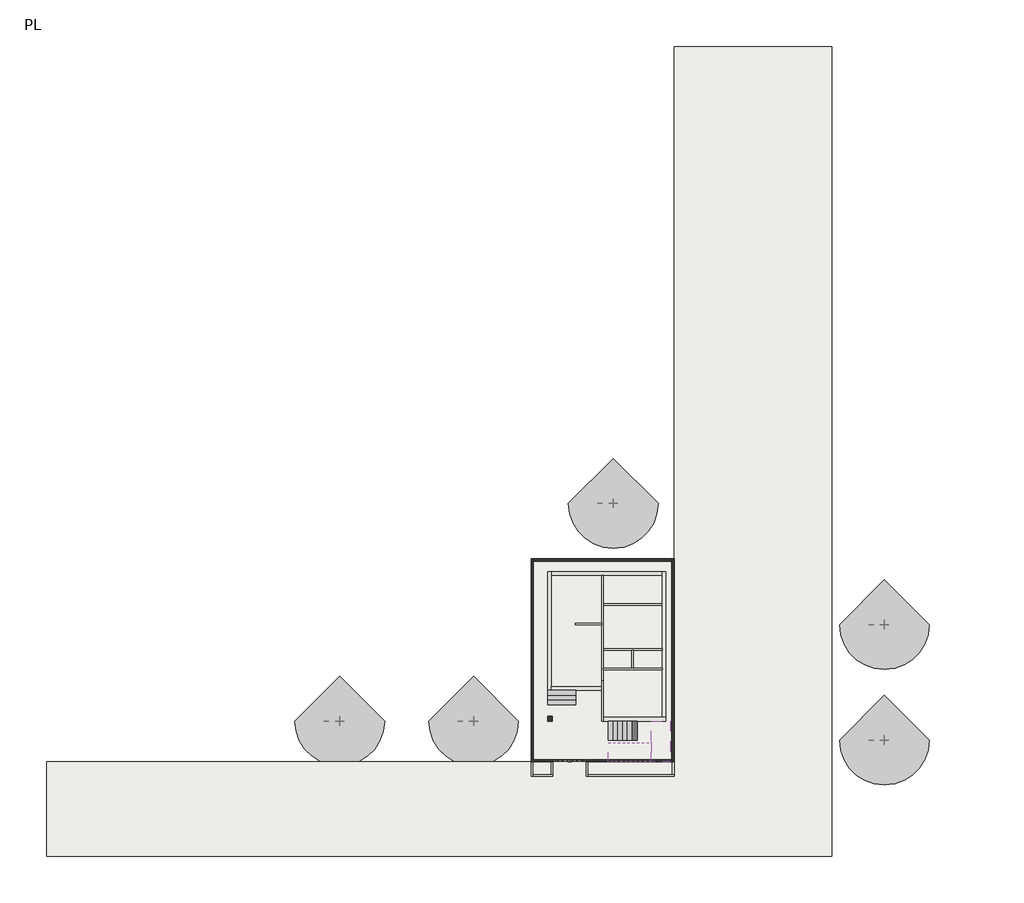
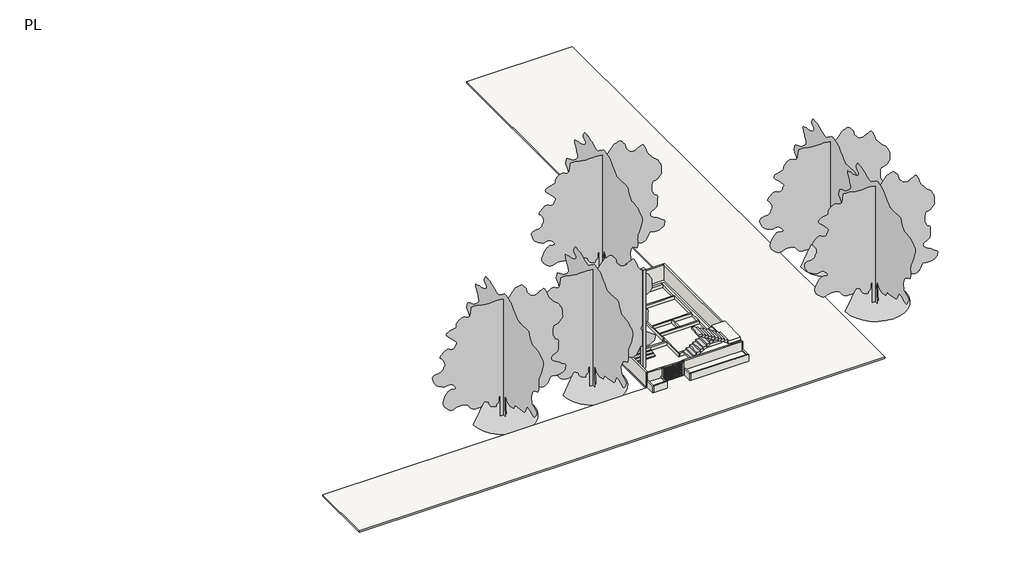
# One storey, incomplete: 23 walls, 5 geographic elements, 5 proxies, 4 slabs, 3 stair flights, 1 column.
"""IFC4 building model written with IfcOpenShell, lengths in millimetres."""

from ifc_helpers import new_model, si_unit, frame, origin, origin_with_axes, place, context, project, spatial, polyline, outline, extrude, faceted_brep, transform, mapped, element, save
from components import generic_models_1_generic_models_1_5ca79dfd, generic_models_2_generic_models_2_e4755291, generic_models_3_generic_models_1_2aceec8a, generic_models_4_generic_models_2_2859856a, generic_models_5_generic_models_5_3b624c68, m_concrete_square_column_300_x_300mm_500808f7, m_rpc_tree_fall_scarlet_oak_12_5_meters_78a4568a

model = new_model("IFC4")

# Units and contexts
model_context = context("Model", 3, world=origin())
ifc_project = project(units=[si_unit("LENGTHUNIT", "METRE", prefix="MILLI")], contexts=[model_context])

# Site, building, storey
site = spatial("IfcSite", under=ifc_project)
building = spatial("IfcBuilding", under=site)
storey = spatial("IfcBuildingStorey", under=building, Name="PL", Elevation=-457.2)

# Proxies
placement = place(None, origin())
generic_models_1_generic_models_1_shape = generic_models_1_generic_models_1_5ca79dfd(model_context)
element("IfcBuildingElementProxy", 1, Name="Generic Models 1 : Generic Models 1", ObjectType="Generic Models 1 : Generic Models 1", at=placement, inside=storey, context=model_context, shape_type="MappedRepresentation", body=[
    mapped(generic_models_1_generic_models_1_shape, transform((160.0, -777.2092348, 0.0), x_axis=(1.0, 0.0, 0.0), y_axis=(0.0, 1.0, 0.0), z_axis=(0.0, 0.0, 1.0))),
])
generic_models_2_generic_models_2_shape = generic_models_2_generic_models_2_e4755291(model_context)
element("IfcBuildingElementProxy", 2, Name="Generic Models 2 : Generic Models 2", ObjectType="Generic Models 2 : Generic Models 2", at=placement, inside=storey, context=model_context, shape_type="MappedRepresentation", body=[
    mapped(generic_models_2_generic_models_2_shape, transform((0.0, -777.2092348, 0.0), x_axis=(1.0, 0.0, 0.0), y_axis=(0.0, 1.0, 0.0), z_axis=(0.0, 0.0, 1.0))),
])
generic_models_3_generic_models_1_shape = generic_models_3_generic_models_1_2aceec8a(model_context)
element("IfcBuildingElementProxy", 3, Name="Generic Models 3 : Generic Models 1", ObjectType="Generic Models 3 : Generic Models 1", at=placement, inside=storey, context=model_context, shape_type="MappedRepresentation", body=[
    mapped(generic_models_3_generic_models_1_shape, transform((152.4, -777.2092348, 0.0), x_axis=(1.0, 0.0, 0.0), y_axis=(0.0, 1.0, 0.0), z_axis=(0.0, 0.0, 1.0))),
])
generic_models_4_generic_models_2_shape = generic_models_4_generic_models_2_2859856a(model_context)
element("IfcBuildingElementProxy", 4, Name="Generic Models 4 : Generic Models 2", ObjectType="Generic Models 4 : Generic Models 2", at=placement, inside=storey, context=model_context, shape_type="MappedRepresentation", body=[
    mapped(generic_models_4_generic_models_2_shape, transform((140.0, -777.2092348, 0.0), x_axis=(1.0, 0.0, 0.0), y_axis=(0.0, 1.0, 0.0), z_axis=(0.0, 0.0, 1.0))),
])
generic_models_5_generic_models_5_shape = generic_models_5_generic_models_5_3b624c68(model_context)
element("IfcBuildingElementProxy", 5, Name="Generic Models 5 : Generic Models 5", ObjectType="Generic Models 5 : Generic Models 5", at=placement, inside=storey, context=model_context, shape_type="MappedRepresentation", body=[
    mapped(generic_models_5_generic_models_5_shape, transform((0.0, 0.0, 0.0), x_axis=(1.0, 0.0, 0.0), y_axis=(0.0, 1.0, 0.0), z_axis=(0.0, 0.0, 1.0))),
])

# Column
m_concrete_square_column_300_x_300mm_shape = m_concrete_square_column_300_x_300mm_500808f7(model_context)
element("IfcColumn", 6, ObjectType="M_Concrete-Square-Column : 300 x 300mm", at=placement, inside=storey, context=model_context, shape_type="MappedRepresentation", body=[
    mapped(m_concrete_square_column_300_x_300mm_shape, transform((-3494.8544048, -4265.8648653, 0.0), x_axis=(1.0, 0.0, 0.0), y_axis=(0.0, 1.0, 0.0), z_axis=(0.0, 0.0, 1.0))),
])

# Geographic elements
m_rpc_tree_fall_scarlet_oak_12_5_meters_shape = m_rpc_tree_fall_scarlet_oak_12_5_meters_78a4568a(model_context)
element("IfcGeographicElement", 7, ObjectType="M_RPC Tree - Fall : Scarlet Oak - 12.5 Meters", at=placement, inside=storey, context=model_context, shape_type="MappedRepresentation", body=[
    mapped(m_rpc_tree_fall_scarlet_oak_12_5_meters_shape, transform((-8369.2544048, -4415.8648653, -457.2), x_axis=(1.0, 0.0, 0.0), y_axis=(0.0, 1.0, 0.0), z_axis=(0.0, 0.0, 1.0))),
])
element("IfcGeographicElement", 8, ObjectType="M_RPC Tree - Fall : Scarlet Oak - 12.5 Meters", at=placement, inside=storey, context=model_context, shape_type="MappedRepresentation", body=[
    mapped(m_rpc_tree_fall_scarlet_oak_12_5_meters_shape, transform((-16903.6544048, -4415.8648653, -457.2), x_axis=(1.0, 0.0, 0.0), y_axis=(0.0, 1.0, 0.0), z_axis=(0.0, 0.0, 1.0))),
])
element("IfcGeographicElement", 9, ObjectType="M_RPC Tree - Fall : Scarlet Oak - 12.5 Meters", at=placement, inside=storey, context=model_context, shape_type="MappedRepresentation", body=[
    mapped(m_rpc_tree_fall_scarlet_oak_12_5_meters_shape, transform((17818.1455952, -5635.0648653, -457.2), x_axis=(1.0, 0.0, 0.0), y_axis=(0.0, 1.0, 0.0), z_axis=(0.0, 0.0, 1.0))),
])
element("IfcGeographicElement", 10, ObjectType="M_RPC Tree - Fall : Scarlet Oak - 12.5 Meters", at=placement, inside=storey, context=model_context, shape_type="MappedRepresentation", body=[
    mapped(m_rpc_tree_fall_scarlet_oak_12_5_meters_shape, transform((17818.1455952, 1730.9351347, -457.2), x_axis=(1.0, 0.0, 0.0), y_axis=(0.0, 1.0, 0.0), z_axis=(0.0, 0.0, 1.0))),
])
element("IfcGeographicElement", 11, ObjectType="M_RPC Tree - Fall : Scarlet Oak - 12.5 Meters", at=placement, inside=storey, context=model_context, shape_type="MappedRepresentation", body=[
    mapped(m_rpc_tree_fall_scarlet_oak_12_5_meters_shape, transform((532.9027938, 9457.3072301, -457.2), x_axis=(1.0, 0.0, 0.0), y_axis=(0.0, 1.0, 0.0), z_axis=(0.0, 0.0, 1.0))),
])

# Slabs
element("IfcSlab", 12, ObjectType="300mm Thickness", at=placement, inside=storey, context=model_context, shape_type="Brep", body=[
    faceted_brep([(2959.1455952, -4415.8648653, 1612.2315789), (2959.1455952, -5635.0648653, 1612.2315789), (2959.1455952, -5787.4648653, 1612.2315789), (2959.1455952, -7006.6648653, 1612.2315789), (3177.9478897, -7006.6648653, 1612.2315789), (4178.3455952, -7006.6648653, 1612.2315789), (4178.3455952, -4415.8648653, 1612.2315789), (3045.1433006, -4415.8648653, 1612.2315789), (2959.1455952, -4415.8648653, 1435.7684211), (2959.1455952, -4415.8648653, 1262.4434337), (2959.1455952, -5635.0648653, 1262.4434337), (2959.1455952, -5635.0648653, 1312.2315789), (2959.1455952, -5787.4648653, 1312.2315789), (2959.1455952, -5787.4648653, 1438.9065916), (2959.1455952, -7006.6648653, 1438.9065916), (3177.9478897, -7006.6648653, 1312.2315789), (4178.3455952, -7006.6648653, 1312.2315789), (4178.3455952, -4415.8648653, 1312.2315789), (3045.1433006, -4415.8648653, 1312.2315789), (3177.9478897, -5787.4648653, 1312.2315789), (3045.1433006, -5635.0648653, 1312.2315789)], [[[0, 1, 2, 3, 4, 5, 6, 7]], [[1, 0, 8, 9, 10, 11]], [[2, 1, 11, 12, 13]], [[3, 2, 13, 14]], [[3, 14, 15, 16, 5, 4]], [[6, 5, 16, 17]], [[9, 8, 0, 7, 6, 17, 18]], [[19, 12, 11, 20, 18, 17, 16, 15]], [[12, 19, 13]], [[18, 20, 10, 9]], [[20, 11, 10]], [[19, 15, 14, 13]]]),
])
element("IfcSlab", 13, ObjectType="6\" floor", at=placement, inside=storey, context=model_context, shape_type="SweptSolid", body=[
    extrude(outline(polyline([(4406.9455952, 5921.9351347), (4406.9455952, -7021.8741001), (-4711.6544048, -7021.8741001), (-4711.6544048, 5921.9351347), (4406.9455952, 5921.9351347)])), frame((0.0, 0.0, -609.6), z_axis=(0.0, 0.0, 1.0), x_axis=(1.0, 0.0, 0.0)), (0.0, 0.0, 1.0), 152.4),
])
element("IfcSlab", 14, ObjectType="6\" floor", at=placement, inside=storey, context=model_context, shape_type="SweptSolid", body=[
    extrude(outline(polyline([(4406.9455952, -7021.8741001), (4406.9455952, 38578.1258999), (14465.3455952, 38578.1258999), (14465.3455952, -5401.8741001), (14465.3455952, -13021.8741001), (-35593.0544048, -13021.8741001), (-35593.0544048, -7021.8741001), (4406.9455952, -7021.8741001)])), frame((0.0, 0.0, -533.4), z_axis=(0.0, 0.0, 1.0), x_axis=(1.0, 0.0, 0.0)), (0.0, 0.0, 1.0), 152.4),
])
element("IfcSlab", 15, ObjectType="6\" floor 2", at=placement, inside=storey, context=model_context, shape_type="SweptSolid", body=[
    extrude(outline(polyline([(-3416.2544048, -7021.8741001), (-3416.2544048, -7834.6741001), (-4610.0544048, -7834.6741001), (-4610.0544048, -7021.8741001), (-3416.2544048, -7021.8741001)])), origin_with_axes(), (0.0, 0.0, 1.0), 152.4),
    extrude(outline(polyline([(4305.3455952, -7021.8741001), (4305.3455952, -7834.6741001), (-1079.4544048, -7834.6741001), (-1079.4544048, -7021.8741001), (4305.3455952, -7021.8741001)])), origin_with_axes(), (0.0, 0.0, 1.0), 152.4),
])

# Stair flights
element("IfcStairFlight", 16, ObjectType="150mm Depth", at=placement, inside=storey, context=model_context, shape_type="Brep", body=[
    faceted_brep([(-3644.8544048, -3069.6648653, -342.9), (-3644.8544048, -3374.4648653, -342.9), (-1854.2524777, -3374.4648653, -342.9), (-1854.2524777, -3069.6648653, -342.9), (-3644.8544048, -3069.6648653, -457.2), (-3644.8544048, -3374.4648653, -457.2), (-1854.2524777, -3374.4648653, -457.2), (-1854.2524777, -3069.6648653, -457.2), (-3644.8544048, -2764.8648653, -228.6), (-3644.8544048, -3069.6648653, -228.6), (-1854.2524777, -3069.6648653, -228.6), (-1854.2524777, -2764.8648653, -228.6), (-3644.8544048, -2764.8648653, -388.8000702), (-3644.8544048, -2947.264678, -457.2), (-1854.2524777, -2947.264678, -457.2), (-1854.2524777, -2764.8648653, -388.8000702), (-3644.8544048, -2460.0648653, -114.3), (-3644.8544048, -2764.8648653, -114.3), (-1854.2524777, -2764.8648653, -114.3), (-1854.2524777, -2460.0648653, -114.3), (-3644.8544048, -2460.0648653, -274.5000702), (-1854.2524777, -2460.0648653, -274.5000702)], [[[0, 1, 2, 3]], [[1, 0, 4, 5]], [[2, 1, 5, 6]], [[3, 2, 6, 7]], [[8, 9, 10, 11]], [[4, 0, 9, 8, 12, 13]], [[0, 3, 10, 9]], [[3, 7, 14, 15, 11, 10]], [[16, 17, 18, 19]], [[17, 16, 20, 12, 8]], [[8, 11, 18, 17]], [[19, 18, 11, 15, 21]], [[16, 19, 21, 20]], [[5, 4, 13, 14, 7, 6]], [[14, 13, 12, 20, 21, 15]]]),
])
element("IfcStairFlight", 17, ObjectType="150mm Depth", at=placement, inside=storey, context=model_context, shape_type="Brep", body=[
    faceted_brep([(520.7455952, -4415.8648653, 24.0631579), (215.9455952, -4415.8648653, 24.0631579), (215.9455952, -5635.0648653, 24.0631579), (520.7455952, -5635.0648653, 24.0631579), (520.7455952, -4415.8648653, -149.2618295), (515.3251188, -4415.8648653, -152.4), (215.9455952, -4415.8648653, -152.4), (215.9455952, -5635.0648653, -152.4), (515.3251188, -5635.0648653, -152.4), (520.7455952, -5635.0648653, -149.2618295), (825.5455952, -4415.8648653, 200.5263158), (520.7455952, -4415.8648653, 200.5263158), (520.7455952, -5635.0648653, 200.5263158), (825.5455952, -5635.0648653, 200.5263158), (825.5455952, -4415.8648653, 27.2013284), (825.5455952, -5635.0648653, 27.2013284), (1130.3455952, -4415.8648653, 376.9894737), (825.5455952, -4415.8648653, 376.9894737), (825.5455952, -5635.0648653, 376.9894737), (1130.3455952, -5635.0648653, 376.9894737), (1130.3455952, -4415.8648653, 203.6644863), (1130.3455952, -5635.0648653, 203.6644863), (1435.1455952, -4415.8648653, 553.4526316), (1130.3455952, -4415.8648653, 553.4526316), (1130.3455952, -5635.0648653, 553.4526316), (1435.1455952, -5635.0648653, 553.4526316), (1435.1455952, -4415.8648653, 380.1276442), (1435.1455952, -5635.0648653, 380.1276442), (1739.9455952, -4415.8648653, 729.9157895), (1435.1455952, -4415.8648653, 729.9157895), (1435.1455952, -5635.0648653, 729.9157895), (1739.9455952, -5635.0648653, 729.9157895), (1739.9455952, -4415.8648653, 556.5908021), (1739.9455952, -5635.0648653, 556.5908021), (2044.7455952, -4415.8648653, 906.3789474), (1739.9455952, -4415.8648653, 906.3789474), (1739.9455952, -5635.0648653, 906.3789474), (2044.7455952, -5635.0648653, 906.3789474), (2044.7455952, -4415.8648653, 733.05396), (2044.7455952, -5635.0648653, 733.05396), (2349.5455952, -4415.8648653, 1082.8421053), (2044.7455952, -4415.8648653, 1082.8421053), (2044.7455952, -5635.0648653, 1082.8421053), (2349.5455952, -5635.0648653, 1082.8421053), (2349.5455952, -4415.8648653, 909.5171179), (2349.5455952, -5635.0648653, 909.5171179), (2654.3455952, -4415.8648653, 1259.3052632), (2349.5455952, -4415.8648653, 1259.3052632), (2349.5455952, -5635.0648653, 1259.3052632), (2654.3455952, -5635.0648653, 1259.3052632), (2654.3455952, -4415.8648653, 1085.9802758), (2654.3455952, -5635.0648653, 1085.9802758), (2959.1455952, -4415.8648653, 1435.7684211), (2654.3455952, -4415.8648653, 1435.7684211), (2654.3455952, -5635.0648653, 1435.7684211), (2959.1455952, -5635.0648653, 1435.7684211), (2959.1455952, -4415.8648653, 1262.4434337), (2959.1455952, -5635.0648653, 1262.4434337), (2959.1455952, -5635.0648653, 1312.2315789)], [[[0, 1, 2, 3]], [[1, 0, 4, 5, 6]], [[2, 1, 6, 7]], [[3, 2, 7, 8, 9]], [[10, 11, 12, 13]], [[11, 10, 14, 4, 0]], [[0, 3, 12, 11]], [[13, 12, 3, 9, 15]], [[16, 17, 18, 19]], [[17, 16, 20, 14, 10]], [[10, 13, 18, 17]], [[19, 18, 13, 15, 21]], [[22, 23, 24, 25]], [[23, 22, 26, 20, 16]], [[16, 19, 24, 23]], [[25, 24, 19, 21, 27]], [[28, 29, 30, 31]], [[29, 28, 32, 26, 22]], [[22, 25, 30, 29]], [[31, 30, 25, 27, 33]], [[34, 35, 36, 37]], [[35, 34, 38, 32, 28]], [[28, 31, 36, 35]], [[37, 36, 31, 33, 39]], [[40, 41, 42, 43]], [[41, 40, 44, 38, 34]], [[34, 37, 42, 41]], [[43, 42, 37, 39, 45]], [[46, 47, 48, 49]], [[47, 46, 50, 44, 40]], [[40, 43, 48, 47]], [[49, 48, 43, 45, 51]], [[52, 53, 54, 55]], [[53, 52, 56, 50, 46]], [[46, 49, 54, 53]], [[55, 54, 49, 51, 57, 58]], [[52, 55, 58, 57, 56]], [[7, 6, 5, 8]], [[8, 5, 4, 14, 20, 26, 32, 38, 44, 50, 56, 57, 51, 45, 39, 33, 27, 21, 15, 9]]]),
])
element("IfcStairFlight", 18, ObjectType="150mm Depth", at=placement, inside=storey, context=model_context, shape_type="Brep", body=[
    faceted_brep([(2654.3455952, -7006.6648653, 1788.6947368), (2959.1455952, -7006.6648653, 1788.6947368), (2959.1455952, -5787.4648653, 1788.6947368), (2654.3455952, -5787.4648653, 1788.6947368), (2654.3455952, -7006.6648653, 1615.3697495), (2959.1455952, -7006.6648653, 1438.9065916), (2959.1455952, -7006.6648653, 1612.2315789), (2959.1455952, -5787.4648653, 1438.9065916), (2654.3455952, -5787.4648653, 1615.3697495), (2349.5455952, -7006.6648653, 1965.1578947), (2654.3455952, -7006.6648653, 1965.1578947), (2654.3455952, -5787.4648653, 1965.1578947), (2349.5455952, -5787.4648653, 1965.1578947), (2349.5455952, -7006.6648653, 1791.8329074), (2349.5455952, -5787.4648653, 1791.8329074), (2044.7455952, -7006.6648653, 2141.6210526), (2349.5455952, -7006.6648653, 2141.6210526), (2349.5455952, -5787.4648653, 2141.6210526), (2044.7455952, -5787.4648653, 2141.6210526), (2044.7455952, -7006.6648653, 1968.2960653), (2044.7455952, -5787.4648653, 1968.2960653), (1739.9455952, -7006.6648653, 2318.0842105), (2044.7455952, -7006.6648653, 2318.0842105), (2044.7455952, -5787.4648653, 2318.0842105), (1739.9455952, -5787.4648653, 2318.0842105), (1739.9455952, -7006.6648653, 2144.7592232), (1739.9455952, -5787.4648653, 2144.7592232), (1435.1455952, -7006.6648653, 2494.5473684), (1739.9455952, -7006.6648653, 2494.5473684), (1739.9455952, -5787.4648653, 2494.5473684), (1435.1455952, -5787.4648653, 2494.5473684), (1435.1455952, -7006.6648653, 2321.2223811), (1435.1455952, -5787.4648653, 2321.2223811), (1130.3455952, -7006.6648653, 2671.0105263), (1435.1455952, -7006.6648653, 2671.0105263), (1435.1455952, -5787.4648653, 2671.0105263), (1130.3455952, -5787.4648653, 2671.0105263), (1130.3455952, -7006.6648653, 2497.6855389), (1130.3455952, -5787.4648653, 2497.6855389), (825.5455952, -7006.6648653, 2847.4736842), (1130.3455952, -7006.6648653, 2847.4736842), (1130.3455952, -5787.4648653, 2847.4736842), (825.5455952, -5787.4648653, 2847.4736842), (825.5455952, -7006.6648653, 2674.1486968), (825.5455952, -5787.4648653, 2674.1486968), (520.7455952, -7006.6648653, 3023.9368421), (825.5455952, -7006.6648653, 3023.9368421), (825.5455952, -5787.4648653, 3023.9368421), (520.7455952, -5787.4648653, 3023.9368421), (520.7455952, -7006.6648653, 2850.6118547), (520.7455952, -5787.4648653, 2850.6118547), (215.9455952, -7006.6648653, 3200.4), (520.7455952, -7006.6648653, 3200.4), (520.7455952, -5787.4648653, 3200.4), (215.9455952, -5787.4648653, 3200.4), (215.9455952, -7006.6648653, 3027.0750126), (215.9455952, -5787.4648653, 3027.0750126)], [[[0, 1, 2, 3]], [[1, 0, 4, 5, 6]], [[2, 1, 6, 5, 7]], [[3, 2, 7, 8]], [[9, 10, 11, 12]], [[10, 9, 13, 4, 0]], [[11, 10, 0, 3]], [[12, 11, 3, 8, 14]], [[15, 16, 17, 18]], [[16, 15, 19, 13, 9]], [[17, 16, 9, 12]], [[18, 17, 12, 14, 20]], [[21, 22, 23, 24]], [[22, 21, 25, 19, 15]], [[23, 22, 15, 18]], [[24, 23, 18, 20, 26]], [[27, 28, 29, 30]], [[28, 27, 31, 25, 21]], [[29, 28, 21, 24]], [[30, 29, 24, 26, 32]], [[33, 34, 35, 36]], [[34, 33, 37, 31, 27]], [[35, 34, 27, 30]], [[36, 35, 30, 32, 38]], [[39, 40, 41, 42]], [[40, 39, 43, 37, 33]], [[41, 40, 33, 36]], [[42, 41, 36, 38, 44]], [[45, 46, 47, 48]], [[46, 45, 49, 43, 39]], [[47, 46, 39, 42]], [[48, 47, 42, 44, 50]], [[51, 52, 53, 54]], [[52, 51, 55, 49, 45]], [[53, 52, 45, 48]], [[54, 53, 48, 50, 56]], [[51, 54, 56, 55]], [[5, 4, 13, 19, 25, 31, 37, 43, 49, 55, 56, 50, 44, 38, 32, 26, 20, 14, 8, 7]]]),
])

# Walls
element("IfcWall", 19, ObjectType="4\" wall", at=placement, inside=storey, context=model_context, shape_type="Brep", body=[
    faceted_brep([(-215.8544048, -1845.1648653, -457.2), (-215.8544048, -2231.4648653, -457.2), (-215.8544048, -2460.0648653, -457.2), (-215.8544048, -4415.8648653, -457.2), (-215.8544048, -4415.8648653, -152.4), (-215.8544048, -2460.0648653, -152.4), (-215.8544048, -2231.4648653, -152.4), (-215.8544048, -1845.1648653, -152.4), (-114.2544048, -1845.1648653, -457.2), (-114.2544048, -1845.1648653, -152.4), (-114.2544048, -4187.2648653, -152.4), (-114.2544048, -4415.8648653, -152.4), (-114.2544048, -4415.8648653, -457.2), (-114.2544048, -4187.2648653, -457.2)], [[[0, 1, 2, 3, 4, 5, 6, 7]], [[8, 9, 10, 11, 12, 13]], [[3, 2, 1, 0, 8, 13, 12]], [[7, 6, 5, 4, 11, 10, 9]], [[0, 7, 9, 8]], [[4, 3, 12, 11]]]),
])
element("IfcWall", 20, ObjectType="4\" wall", at=placement, inside=storey, context=model_context, shape_type="Brep", body=[
    faceted_brep([(-215.8544048, 4880.5351347, -457.2), (-215.8544048, 1832.5351347, -457.2), (-215.8544048, 1730.9351347, -457.2), (-215.8544048, -1845.1648653, -457.2), (-215.8544048, -1845.1648653, -152.4), (-215.8544048, 1730.9351347, -152.4), (-215.8544048, 1832.5351347, -152.4), (-215.8544048, 4880.5351347, -152.4), (-114.2544048, 4880.5351347, -457.2), (-114.2544048, 4880.5351347, -152.4), (-114.2544048, 3051.7351347, -152.4), (-114.2544048, 2950.1351347, -152.4), (-114.2544048, 206.9351347, -152.4), (-114.2544048, 105.3351347, -152.4), (-114.2544048, -1037.6648653, -152.4), (-114.2544048, -1139.2648653, -152.4), (-114.2544048, -1845.1648653, -152.4), (-114.2544048, -1845.1648653, -457.2), (-114.2544048, -1139.2648653, -457.2), (-114.2544048, -1037.6648653, -457.2), (-114.2544048, 105.3351347, -457.2), (-114.2544048, 206.9351347, -457.2), (-114.2544048, 2950.1351347, -457.2), (-114.2544048, 3051.7351347, -457.2)], [[[0, 1, 2, 3, 4, 5, 6, 7]], [[8, 9, 10, 11, 12, 13, 14, 15, 16, 17, 18, 19, 20, 21, 22, 23]], [[3, 2, 1, 0, 8, 23, 22, 21, 20, 19, 18, 17]], [[4, 3, 17, 16]], [[7, 6, 5, 4, 16, 15, 14, 13, 12, 11, 10, 9]], [[0, 7, 9, 8]]]),
])
element("IfcWall", 21, ObjectType="4\" wall", at=placement, inside=storey, context=model_context, shape_type="Brep", body=[
    faceted_brep([(-114.2544048, -1139.2648653, -457.2), (3644.9455952, -1139.2648653, -457.2), (3644.9455952, -1139.2648653, -152.4), (-114.2544048, -1139.2648653, -152.4), (-114.2544048, -1037.6648653, -457.2), (-114.2544048, -1037.6648653, -152.4), (1714.5455952, -1037.6648653, -152.4), (1816.1455952, -1037.6648653, -152.4), (3644.9455952, -1037.6648653, -152.4), (3644.9455952, -1037.6648653, -457.2), (1816.1455952, -1037.6648653, -457.2), (1714.5455952, -1037.6648653, -457.2)], [[[0, 1, 2, 3]], [[4, 5, 6, 7, 8, 9, 10, 11]], [[1, 0, 4, 11, 10, 9]], [[3, 2, 8, 7, 6, 5]], [[2, 1, 9, 8]], [[0, 3, 5, 4]]]),
])
element("IfcWall", 22, ObjectType="4\" wall", at=placement, inside=storey, context=model_context, shape_type="Brep", body=[
    faceted_brep([(3644.9455952, 206.9351347, -457.2), (-114.2544048, 206.9351347, -457.2), (-114.2544048, 206.9351347, -152.4), (3644.9455952, 206.9351347, -152.4), (3644.9455952, 105.3351347, -457.2), (3644.9455952, 105.3351347, -152.4), (1816.1455952, 105.3351347, -152.4), (1714.5455952, 105.3351347, -152.4), (-114.2544048, 105.3351347, -152.4), (-114.2544048, 105.3351347, -457.2), (1714.5455952, 105.3351347, -457.2), (1816.1455952, 105.3351347, -457.2)], [[[0, 1, 2, 3]], [[4, 5, 6, 7, 8, 9, 10, 11]], [[1, 0, 4, 11, 10, 9]], [[3, 2, 8, 7, 6, 5]], [[0, 3, 5, 4]], [[2, 1, 9, 8]]]),
])
element("IfcWall", 23, ObjectType="4\" wall", at=placement, inside=storey, context=model_context, shape_type="SweptSolid", body=[
    extrude(outline(polyline([(-215.8544048, 1730.9351347), (-1892.2544048, 1730.9351347), (-1892.2544048, 1832.5351347), (-215.8544048, 1832.5351347), (-215.8544048, 1730.9351347)])), frame((0.0, 0.0, -457.2), z_axis=(0.0, 0.0, 1.0), x_axis=(1.0, 0.0, 0.0)), (0.0, 0.0, 1.0), 304.8),
])
element("IfcWall", 24, ObjectType="4\" wall", at=placement, inside=storey, context=model_context, shape_type="SweptSolid", body=[
    extrude(outline(polyline([(-114.2544048, 3051.7351347), (3644.9455952, 3051.7351347), (3644.9455952, 2950.1351347), (-114.2544048, 2950.1351347), (-114.2544048, 3051.7351347)])), frame((0.0, 0.0, -457.2), z_axis=(0.0, 0.0, 1.0), x_axis=(1.0, 0.0, 0.0)), (0.0, 0.0, 1.0), 304.8),
])
element("IfcWall", 25, ObjectType="4\" wall", at=placement, inside=storey, context=model_context, shape_type="SweptSolid", body=[
    extrude(outline(polyline([(1714.5455952, -1037.6648653), (1714.5455952, 105.3351347), (1816.1455952, 105.3351347), (1816.1455952, -1037.6648653), (1714.5455952, -1037.6648653)])), frame((0.0, 0.0, -457.2), z_axis=(0.0, 0.0, 1.0), x_axis=(1.0, 0.0, 0.0)), (0.0, 0.0, 1.0), 304.8),
])
element("IfcWall", 26, ObjectType="4\" wall", at=placement, inside=storey, context=model_context, shape_type="Brep", body=[
    faceted_brep([(-4711.6544048, -7021.8741001, -457.2), (-4711.6544048, -7936.2741001, -457.2), (-4711.6544048, -7936.2741001, 304.8), (-4711.6544048, -7021.8741001, 304.8), (-4610.0544048, -7021.8741001, -457.2), (-4610.0544048, -7021.8741001, 304.8), (-4610.0544048, -7834.6741001, 304.8), (-4610.0544048, -7936.2741001, 304.8), (-4610.0544048, -7936.2741001, -457.2), (-4610.0544048, -7834.6741001, -457.2)], [[[0, 1, 2, 3]], [[4, 5, 6, 7, 8, 9]], [[1, 0, 4, 9, 8]], [[3, 2, 7, 6, 5]], [[0, 3, 5, 4]], [[2, 1, 8, 7]]]),
])
element("IfcWall", 27, ObjectType="4\" wall", at=placement, inside=storey, context=model_context, shape_type="Brep", body=[
    faceted_brep([(-4610.0544048, -7936.2741001, -457.2), (-3314.6544048, -7936.2741001, -457.2), (-3314.6544048, -7936.2741001, 304.8), (-4610.0544048, -7936.2741001, 304.8), (-4610.0544048, -7834.6741001, -457.2), (-4610.0544048, -7834.6741001, 304.8), (-3416.2544048, -7834.6741001, 304.8), (-3314.6544048, -7834.6741001, 304.8), (-3314.6544048, -7834.6741001, -457.2), (-3416.2544048, -7834.6741001, -457.2)], [[[0, 1, 2, 3]], [[4, 5, 6, 7, 8, 9]], [[1, 0, 4, 9, 8]], [[3, 2, 7, 6, 5]], [[0, 3, 5, 4]], [[2, 1, 8, 7]]]),
])
element("IfcWall", 28, ObjectType="4\" wall", at=placement, inside=storey, context=model_context, shape_type="SweptSolid", body=[
    extrude(outline(polyline([(-3314.6544048, -7021.8741001), (-3314.6544048, -7834.6741001), (-3416.2544048, -7834.6741001), (-3416.2544048, -7021.8741001), (-3314.6544048, -7021.8741001)])), frame((0.0, 0.0, -457.2), z_axis=(0.0, 0.0, 1.0), x_axis=(1.0, 0.0, 0.0)), (0.0, 0.0, 1.0), 762.0),
])
element("IfcWall", 29, ObjectType="4\" wall", at=placement, inside=storey, context=model_context, shape_type="Brep", body=[
    faceted_brep([(-1181.0544048, -7021.8741001, -457.2), (-1181.0544048, -7936.2741001, -457.2), (-1181.0544048, -7936.2741001, 304.8), (-1181.0544048, -7021.8741001, 304.8), (-1079.4544048, -7021.8741001, -457.2), (-1079.4544048, -7021.8741001, 304.8), (-1079.4544048, -7834.6741001, 304.8), (-1079.4544048, -7936.2741001, 304.8), (-1079.4544048, -7936.2741001, -457.2), (-1079.4544048, -7834.6741001, -457.2)], [[[0, 1, 2, 3]], [[4, 5, 6, 7, 8, 9]], [[1, 0, 4, 9, 8]], [[3, 2, 7, 6, 5]], [[0, 3, 5, 4]], [[2, 1, 8, 7]]]),
])
element("IfcWall", 30, ObjectType="4\" wall", at=placement, inside=storey, context=model_context, shape_type="Brep", body=[
    faceted_brep([(-1079.4544048, -7936.2741001, -457.2), (4406.9455952, -7936.2741001, -457.2), (4406.9455952, -7936.2741001, 304.8), (-1079.4544048, -7936.2741001, 304.8), (-1079.4544048, -7834.6741001, -457.2), (-1079.4544048, -7834.6741001, 304.8), (4305.3455952, -7834.6741001, 304.8), (4406.9455952, -7834.6741001, 304.8), (4406.9455952, -7834.6741001, -457.2), (4305.3455952, -7834.6741001, -457.2)], [[[0, 1, 2, 3]], [[4, 5, 6, 7, 8, 9]], [[1, 0, 4, 9, 8]], [[3, 2, 7, 6, 5]], [[0, 3, 5, 4]], [[2, 1, 8, 7]]]),
])
element("IfcWall", 31, ObjectType="4\" wall", at=placement, inside=storey, context=model_context, shape_type="SweptSolid", body=[
    extrude(outline(polyline([(4406.9455952, -7021.8741001), (4406.9455952, -7834.6741001), (4305.3455952, -7834.6741001), (4305.3455952, -7021.8741001), (4406.9455952, -7021.8741001)])), frame((0.0, 0.0, -457.2), z_axis=(0.0, 0.0, 1.0), x_axis=(1.0, 0.0, 0.0)), (0.0, 0.0, 1.0), 762.0),
])
element("IfcWall", 32, ObjectType="6\" wall", at=placement, inside=storey, context=model_context, shape_type="Brep", body=[
    faceted_brep([(-4711.6544048, 5921.9351347, -457.2), (-4711.6544048, -6869.4741001, -457.2), (-4711.6544048, -6869.4741001, 1066.8), (-4711.6544048, 5921.9351347, 1066.8), (-4559.2544048, 5921.9351347, -457.2), (-4559.2544048, 5921.9351347, 1066.8), (-4559.2544048, 5769.5351347, 1066.8), (-4559.2544048, -6869.4741001, 1066.8), (-4559.2544048, -6869.4741001, -457.2), (-4559.2544048, 5769.5351347, -457.2)], [[[0, 1, 2, 3]], [[4, 5, 6, 7, 8, 9]], [[1, 0, 4, 9, 8]], [[3, 2, 7, 6, 5]], [[0, 3, 5, 4]], [[1, 8, 7, 2]]]),
])
element("IfcWall", 33, ObjectType="6\" wall", at=placement, inside=storey, context=model_context, shape_type="Brep", body=[
    faceted_brep([(4406.9455952, -7021.8741001, 1066.8), (4406.9455952, -7021.8741001, 304.8), (4406.9455952, -7021.8741001, -457.2), (4406.9455952, 5921.9351347, -457.2), (4406.9455952, 5921.9351347, 1066.8), (4254.5455952, -7021.8741001, -457.2), (4254.5455952, -7021.8741001, 1066.8), (4254.5455952, 5769.5351347, 1066.8), (4254.5455952, 5921.9351347, 1066.8), (4254.5455952, 5921.9351347, -457.2), (4254.5455952, 5769.5351347, -457.2), (4305.3455952, -7021.8741001, -457.2)], [[[0, 1, 2, 3, 4]], [[5, 6, 7, 8, 9, 10]], [[3, 2, 11, 5, 10, 9]], [[0, 4, 8, 7, 6]], [[4, 3, 9, 8]], [[0, 6, 5, 11, 2, 1]]]),
])
element("IfcWall", 34, ObjectType="6\" wall", at=placement, inside=storey, context=model_context, shape_type="SweptSolid", body=[
    extrude(outline(polyline([(-4559.2544048, 5921.9351347), (4254.5455952, 5921.9351347), (4254.5455952, 5769.5351347), (-4559.2544048, 5769.5351347), (-4559.2544048, 5921.9351347)])), frame((0.0, 0.0, -457.2), z_axis=(0.0, 0.0, 1.0), x_axis=(1.0, 0.0, 0.0)), (0.0, 0.0, 1.0), 1524.0),
])
element("IfcWall", 35, ObjectType="6\" wall", at=placement, inside=storey, context=model_context, shape_type="Brep", body=[
    faceted_brep([(-1181.0544048, -7021.8741001, -457.2), (-1079.4544048, -7021.8741001, -457.2), (342.9455952, -7021.8741001, -457.2), (4305.3455952, -7021.8741001, -457.2), (4305.3455952, -7021.8741001, 766.8), (4305.3455952, -7021.8741001, 1066.8), (3924.3455952, -7021.8741001, 1066.8), (2680.8793726, -7021.8741001, 1066.8), (-1181.0544048, -7021.8741001, 1066.8), (-1181.0544048, -7021.8741001, 304.8), (-1181.0544048, -6869.4741001, -457.2), (-1181.0544048, -6869.4741001, 1066.8), (2680.8793726, -6869.4741001, 1066.8), (3924.3455952, -6869.4741001, 1066.8), (4305.3455952, -6869.4741001, 1066.8), (4305.3455952, -6869.4741001, 766.8), (4305.3455952, -6869.4741001, -457.2), (342.9455952, -6869.4741001, -457.2)], [[[0, 1, 2, 3, 4, 5, 6, 7, 8, 9]], [[10, 11, 12, 13, 14, 15, 16, 17]], [[2, 1, 0, 10, 17]], [[8, 7, 12, 11]], [[3, 2, 17, 16]], [[4, 3, 16, 15]], [[5, 4, 15, 14]], [[6, 5, 14, 13]], [[7, 6, 13, 12]], [[0, 9, 8, 11, 10]]]),
])
element("IfcWall", 36, ObjectType="6\" wall", at=placement, inside=storey, context=model_context, shape_type="Brep", body=[
    faceted_brep([(-3314.6544048, -6869.4741001, -457.2), (-4559.2544048, -6869.4741001, -457.2), (-4711.6544048, -6869.4741001, -457.2), (-4711.6544048, -6869.4741001, 1066.8), (-4559.2544048, -6869.4741001, 1066.8), (-3314.6544048, -6869.4741001, 1066.8), (-3314.6544048, -7021.8741001, -457.2), (-3314.6544048, -7021.8741001, 304.8), (-3314.6544048, -7021.8741001, 1066.8), (-4711.6544048, -7021.8741001, 1066.8), (-4711.6544048, -7021.8741001, 304.8), (-4711.6544048, -7021.8741001, -457.2), (-4610.0544048, -7021.8741001, -457.2), (-3416.2544048, -7021.8741001, -457.2)], [[[0, 1, 2, 3, 4, 5]], [[6, 7, 8, 9, 10, 11, 12, 13]], [[2, 1, 0, 6, 13, 12, 11]], [[5, 4, 3, 9, 8]], [[2, 11, 10, 9, 3]], [[0, 5, 8, 7, 6]]]),
])
element("IfcWall", 37, ObjectType="9\" wall", at=placement, inside=storey, context=model_context, shape_type="Brep", body=[
    faceted_brep([(-3644.8544048, 5109.1351347, -457.2), (-3644.8544048, -2460.0648653, -457.2), (-3644.8544048, -2460.0648653, -152.4), (-3644.8544048, 5109.1351347, -152.4), (-3416.2544048, 5109.1351347, -457.2), (-3416.2544048, 5109.1351347, -152.4), (-3416.2544048, 4880.5351347, -152.4), (-3416.2544048, -2231.4648653, -152.4), (-3416.2544048, -2460.0648653, -152.4), (-3416.2544048, -2460.0648653, -457.2), (-3416.2544048, -2231.4648653, -457.2), (-3416.2544048, 4880.5351347, -457.2)], [[[0, 1, 2, 3]], [[4, 5, 6, 7, 8, 9, 10, 11]], [[1, 0, 4, 11, 10, 9]], [[3, 2, 8, 7, 6, 5]], [[2, 1, 9, 8]], [[0, 3, 5, 4]]]),
])
element("IfcWall", 38, ObjectType="9\" wall", at=placement, inside=storey, context=model_context, shape_type="SweptSolid", body=[
    extrude(outline(polyline([(-215.8544048, -2460.0648653), (-3416.2544048, -2460.0648653), (-3416.2544048, -2231.4648653), (-215.8544048, -2231.4648653), (-215.8544048, -2460.0648653)])), frame((0.0, 0.0, -457.2), z_axis=(0.0, 0.0, 1.0), x_axis=(1.0, 0.0, 0.0)), (0.0, 0.0, 1.0), 304.8),
])
element("IfcWall", 39, ObjectType="9\" wall", at=placement, inside=storey, context=model_context, shape_type="Brep", body=[
    faceted_brep([(-114.2544048, -4415.8648653, -457.2), (3873.5455952, -4415.8648653, -457.2), (3873.5455952, -4415.8648653, -152.4), (-114.2544048, -4415.8648653, -152.4), (-114.2544048, -4187.2648653, -457.2), (-114.2544048, -4187.2648653, -152.4), (3644.9455952, -4187.2648653, -152.4), (3873.5455952, -4187.2648653, -152.4), (3873.5455952, -4187.2648653, -457.2), (3644.9455952, -4187.2648653, -457.2)], [[[0, 1, 2, 3]], [[4, 5, 6, 7, 8, 9]], [[1, 0, 4, 9, 8]], [[3, 2, 7, 6, 5]], [[0, 3, 5, 4]], [[2, 1, 8, 7]]]),
])
element("IfcWall", 40, ObjectType="9\" wall", at=placement, inside=storey, context=model_context, shape_type="Brep", body=[
    faceted_brep([(3873.5455952, -4187.2648653, -457.2), (3873.5455952, 5109.1351347, -457.2), (3873.5455952, 5109.1351347, -152.4), (3873.5455952, -4187.2648653, -152.4), (3644.9455952, -4187.2648653, -457.2), (3644.9455952, -4187.2648653, -152.4), (3644.9455952, -1139.2648653, -152.4), (3644.9455952, -1037.6648653, -152.4), (3644.9455952, 105.3351347, -152.4), (3644.9455952, 206.9351347, -152.4), (3644.9455952, 2950.1351347, -152.4), (3644.9455952, 3051.7351347, -152.4), (3644.9455952, 4880.5351347, -152.4), (3644.9455952, 5109.1351347, -152.4), (3644.9455952, 5109.1351347, -457.2), (3644.9455952, 4880.5351347, -457.2), (3644.9455952, 3051.7351347, -457.2), (3644.9455952, 2950.1351347, -457.2), (3644.9455952, 206.9351347, -457.2), (3644.9455952, 105.3351347, -457.2), (3644.9455952, -1037.6648653, -457.2), (3644.9455952, -1139.2648653, -457.2)], [[[0, 1, 2, 3]], [[4, 5, 6, 7, 8, 9, 10, 11, 12, 13, 14, 15, 16, 17, 18, 19, 20, 21]], [[1, 0, 4, 21, 20, 19, 18, 17, 16, 15, 14]], [[3, 2, 13, 12, 11, 10, 9, 8, 7, 6, 5]], [[0, 3, 5, 4]], [[2, 1, 14, 13]]]),
])
element("IfcWall", 41, ObjectType="9\" wall", at=placement, inside=storey, context=model_context, shape_type="Brep", body=[
    faceted_brep([(3644.9455952, 5109.1351347, -457.2), (-3416.2544048, 5109.1351347, -457.2), (-3416.2544048, 5109.1351347, -152.4), (3644.9455952, 5109.1351347, -152.4), (3644.9455952, 4880.5351347, -457.2), (3644.9455952, 4880.5351347, -152.4), (-114.2544048, 4880.5351347, -152.4), (-215.8544048, 4880.5351347, -152.4), (-3416.2544048, 4880.5351347, -152.4), (-3416.2544048, 4880.5351347, -457.2), (-215.8544048, 4880.5351347, -457.2), (-114.2544048, 4880.5351347, -457.2)], [[[0, 1, 2, 3]], [[4, 5, 6, 7, 8, 9, 10, 11]], [[1, 0, 4, 11, 10, 9]], [[3, 2, 8, 7, 6, 5]], [[0, 3, 5, 4]], [[2, 1, 9, 8]]]),
])

save(model, "model.ifc")

# Revit data of these elements
# Type "M_Concrete-Square-Column : 300 x 300mm"
#   b = 0.984252 ft
#   Structural Material [instance default] = Concrete, Cast-in-Place gray
# Type "M_RPC Tree - Fall : Scarlet Oak - 12.5 Meters"
#   built-in parameter 1005198 = "{2, 15},{39, RPC-16-FXGN-QL00-PPP3-E000-ST1L-LVER-AU},{1, 0},{1, 0},{2, 13},{1, 8},{5, Color},{1, 0},{1, 0},{3, 0.8},{3, 0.8},{3, 0.8},{1, 8},{7, BBoxMin},{1, 0},{1, 0},{1, 0},{1, 0},{1, 0},{1, 8},{7, BBoxMax},{1, 0},{1, 0},{1, 0},{1, 0},{1, 0},{2, 11},{9, RPCTypeId},{1, 0},{1, 0},{39, RPC-16-FXGN-QL00-PPP3-E000-ST1L-LVER-AU},{1, 6},{14, RPCPlantHeight},{1, 0},{1, 0},{7, 41.0105},{2, 11},{7, keyword},{1, 0},{1, 0},{39, :RPCs:Fall Trees [General]:Geometry:RPC},{2, 11},{8, category},{1, 0},{1, 0},{20, Fall Trees [General]},{2, 11},{12, LocalizedUID},{1, 0},{1, 0},{18, Scarlet Oak [Fall]},{2, 14},{6, Height},{1, 0},{1, 0},{7, 41.0105},{1, 2},{16, Cast Reflections},{1, 0},{1, 0},{1, 0},{1, 2},{12, Cast Shadows},{1, 0},{1, 0},{1, 1},{1, 2},{9, Lock View},{1, 0},{1, 0},{1, 0},{1, 4},{5, ViewC},{1, 0},{1, 0},{1, 0},{21, assetlibrary_base.fbx},{1, 5},"
#   built-in parameter 1005195 = "RPC-16-FXGN-QL00-PPP3-E000-ST1L-LVER-AU"
#   Type Comments = "Scarlet Oak"
#   Height = 41.010499 ft
#   Default Elevation = 0
# Type "6\" floor"
#   Function = 0
#   Layers, outside or top first: 0.5 ft no material (function 1)
# Type "6\" floor 2"
#   Function = 0
#   Layers, outside or top first: 0.5 ft "Grass" (function 1)
# Type "4\" wall"
#   Layers, outside or top first: 0.333333 ft no material (function 1)
# Type "6\" wall"
#   Layers, outside or top first: 0.5 ft no material (function 1)
# Type "9\" wall"
#   Layers, outside or top first: 0.75 ft no material (function 1)
# Element 1 (IfcBuildingElementProxy, "Generic Models 1 : Generic Models 1")
#   Phase Created = New Construction
# Element 2 (IfcBuildingElementProxy, "Generic Models 2 : Generic Models 2")
#   Phase Created = New Construction
# Element 3 (IfcBuildingElementProxy, "Generic Models 3 : Generic Models 1")
#   Phase Created = New Construction
# Element 4 (IfcBuildingElementProxy, "Generic Models 4 : Generic Models 2")
#   Phase Created = New Construction
# Element 5 (IfcBuildingElementProxy, "Generic Models 5 : Generic Models 5")
#   Phase Created = New Construction
# Element 6 (IfcColumn, "M_Concrete-Square-Column : 300 x 300mm")
#   Structural Material = Concrete, Cast-in-Place gray
#   Phase Created = New Construction
#   Materials on its faces: "Concrete, Cast-in-Place gray"
# Elements 7, 8, 9, 10, 11 (IfcGeographicElement, "M_RPC Tree - Fall : Scarlet Oak - 12.5 Meters")
#   Phase Created = New Construction
# Element 12 (IfcSlab, "300mm Thickness")
#   Phase Created = New Construction
#   Materials on its faces: "Concrete, Cast In Situ"
# Element 13 (IfcSlab, "6\" floor")
#   Height Offset From Level = 0.0 ft
#   Phase Created = New Construction
#   Materials on its faces: "Default Floor"
# Element 14 (IfcSlab, "6\" floor")
#   Height Offset From Level = 0.25 ft
#   Phase Created = New Construction
#   Materials on its faces: "Default Floor", "Asphalt, Bitumen"
# Element 15 (IfcSlab, "6\" floor 2")
#   Height Offset From Level = 2.0 ft
#   Phase Created = New Construction
#   Materials on its faces: "Grass"
# Elements 16, 17, 18 (IfcStairFlight, "150mm Depth")
#   Phase Created = New Construction
#   Materials on its faces: "Concrete, Cast In Situ"
# Elements 19, 20, 21, 22, 23, 24, 25 (IfcWall, "4\" wall")
#   Top Offset = 0.0 ft
#   Base Offset = 0.0 ft
#   Unconnected Height = 1.0 ft
#   wall height = 1.0 ft
#   Phase Created = New Construction
#   Base Constraint = PL
#   Materials on its faces: "Default Wall"
# Elements 26, 27, 28, 29, 30, 31 (IfcWall, "4\" wall")
#   Top Offset = 0.0 ft
#   Base Offset = 0.0 ft
#   Unconnected Height = 2.5 ft
#   wall height = 2.5 ft
#   Phase Created = New Construction
#   Base Constraint = PL
#   Materials on its faces: "Default Wall"
# Elements 32, 33, 34, 35, 36 (IfcWall, "6\" wall")
#   Top Offset = 0.0 ft
#   Base Offset = 0.0 ft
#   Unconnected Height = 5.0 ft
#   wall height = 5.0 ft
#   Phase Created = New Construction
#   Base Constraint = PL
#   Materials on its faces: "Default Wall"
# Elements 37, 38, 39, 40, 41 (IfcWall, "9\" wall")
#   Top Offset = 0.0 ft
#   Base Offset = 0.0 ft
#   Unconnected Height = 1.0 ft
#   wall height = 1.0 ft
#   Phase Created = New Construction
#   Base Constraint = PL
#   Materials on its faces: "Default Wall"
# Materials
#   "Concrete, Cast-in-Place gray": class "Concrete", colour RGB 192 192 192, transparency 0, Description = "Cast-in-place concrete", Cost = 0
#   "Grass": class "Generic", colour RGB 0 185 92, transparency 0, Description = "Physical material.", Cost = 0
#   "Concrete, Cast In Situ": class "Concrete", colour RGB 192 192 192, transparency 0, Description = "physical material", Cost = 0
#   "Default Floor": colour RGB 127 127 127, transparency 0, Cost = 0
#   "Asphalt, Bitumen": class "Generic", colour RGB 155 155 155, transparency 0, Description = "Bituminous roofing material", Cost = 0
#   "Default Wall": colour RGB 128 128 128, transparency 0, Cost = 0
